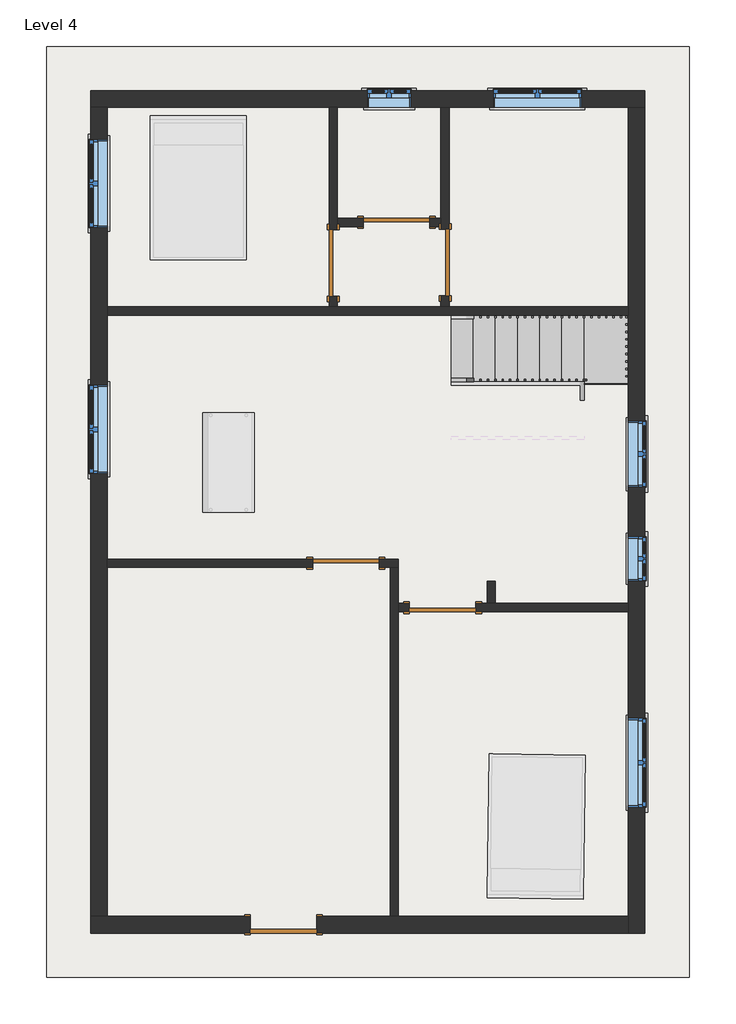
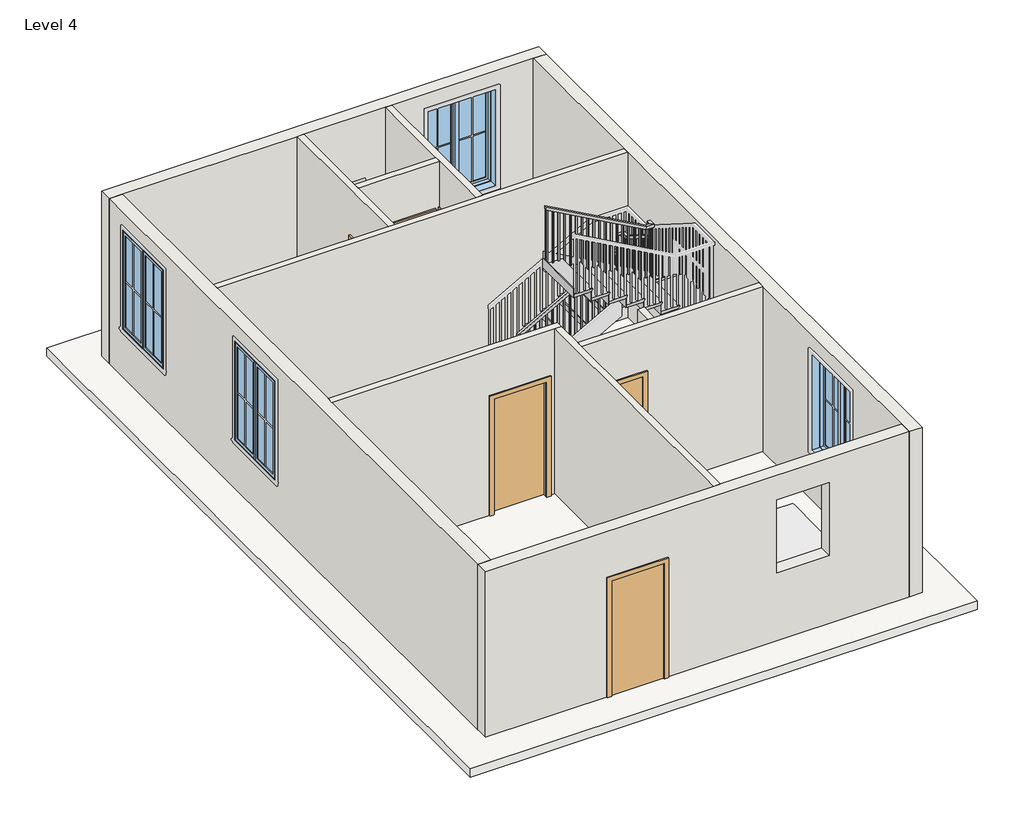
# One storey, part 1 of 2: 12 walls, 7 windows, 6 doors, 1 railing, 1 slab, 1 stair flight.
"""IFC4 building model written with IfcOpenShell, lengths in millimetres."""

from ifc_helpers import new_model, si_unit, frame, origin, place, context, project, spatial, polyline, outline, extrude, faceted_brep, transform, mapped, element, save
from components import door_e5f9f3c4, door_305aa2a5, door_0ca8825f, stair_flight_9a0573e1, window_c417fced, window_79f73a1a, window_6ca1769e

model = new_model("IFC4")

# Units and contexts
model_context = context("Model", 3, world=origin())
ifc_project = project(units=[si_unit("LENGTHUNIT", "METRE", prefix="MILLI")], contexts=[model_context])

# Site, building, storey
site = spatial("IfcSite", under=ifc_project)
building = spatial("IfcBuilding", under=site)
storey = spatial("IfcBuildingStorey", under=building, Name="Level 4", Elevation=9144.0)

# Doors
placement = place(None, origin())
door_shape = door_e5f9f3c4(model_context)
element("IfcDoor", 1, ObjectType="Single-Flush : 36\" x 84\"", at=placement, inside=storey, context=model_context, shape_type="MappedRepresentation", body=[
    mapped(door_shape, transform((5727.7, 12245.5823212, 9144.0), x_axis=(1.0, 0.0, 0.0), y_axis=(0.0, 1.0, 0.0), z_axis=(0.0, 0.0, 1.0))),
])
element("IfcDoor", 2, ObjectType="Single-Flush : 36\" x 84\"", at=placement, inside=storey, context=model_context, shape_type="MappedRepresentation", body=[
    mapped(door_shape, transform((6394.45, 11693.1323212, 9144.0), x_axis=(0.0, -1.0, 0.0), y_axis=(1.0, 0.0, 0.0), z_axis=(0.0, 0.0, 1.0))),
])
element("IfcDoor", 3, ObjectType="Single-Flush : 36\" x 84\"", at=placement, inside=storey, context=model_context, shape_type="MappedRepresentation", body=[
    mapped(door_shape, transform((6362.7, 6949.6823212, 9144.0), x_axis=(-1.0, 0.0, 0.0), y_axis=(0.0, -1.0, 0.0), z_axis=(0.0, 0.0, 1.0))),
])
element("IfcDoor", 4, ObjectType="Single-Flush : 36\" x 84\"", at=placement, inside=storey, context=model_context, shape_type="MappedRepresentation", body=[
    mapped(door_shape, transform((5029.2, 7559.2823212, 9144.0), x_axis=(1.0, 0.0, 0.0), y_axis=(0.0, 1.0, 0.0), z_axis=(0.0, 0.0, 1.0))),
])
door_2_shape = door_305aa2a5(model_context)
element("IfcDoor", 5, ObjectType="Single-Flush : 36\" x 84\"", at=placement, inside=storey, context=model_context, shape_type="MappedRepresentation", body=[
    mapped(door_2_shape, transform((4857.75, 11689.9573212, 9144.0), x_axis=(0.0, -1.0, 0.0), y_axis=(1.0, 0.0, 0.0), z_axis=(0.0, 0.0, 1.0))),
])
door_3_shape = door_0ca8825f(model_context)
element("IfcDoor", 6, ObjectType="Single-Flush : 36\" x 84\"", at=placement, inside=storey, context=model_context, shape_type="MappedRepresentation", body=[
    mapped(door_3_shape, transform((4171.95, 2587.2323212, 9144.0), x_axis=(-1.0, 0.0, 0.0), y_axis=(0.0, -1.0, 0.0), z_axis=(0.0, 0.0, 1.0))),
])

# Railing
element("IfcRailing", 7, ObjectType="Handrail - Rectangular", at=placement, inside=storey, context=model_context, shape_type="SolidModel", body=[
    faceted_brep([(6477.0, 10105.6323212, 10227.7333333), (6477.0, 10105.6323212, 10169.620221), (6477.0, 10054.8323212, 10169.620221), (6477.0, 10054.8323212, 10227.7333333), (8229.6, 10105.6323212, 11201.4), (8280.4, 10105.6323212, 11171.5091099), (8280.4, 10054.8323212, 11171.5091099), (8229.6, 10054.8323212, 11201.4), (8229.6, 10105.6323212, 11461.447619), (8280.4, 10105.6323212, 11410.647619), (8280.4, 10054.8323212, 11410.647619), (8229.6, 10054.8323212, 11461.447619), (8356.6, 10105.6323212, 11461.447619), (8356.6, 10105.6323212, 11410.647619), (8305.8, 10054.8323212, 11410.647619), (8305.8, 10054.8323212, 11461.447619), (8356.6, 9978.6323212, 11461.447619), (8356.6, 9963.8676405, 11410.647619), (8305.8, 9963.8676405, 11410.647619), (8305.8, 9978.6323212, 11461.447619), (8356.6, 9330.9323212, 11872.6857143), (8356.6, 9280.1323212, 11844.7652821), (8305.8, 9280.1323212, 11844.7652821), (8305.8, 9330.9323212, 11872.6857143), (8356.6, 9330.9323212, 12132.7333333), (8356.6, 9280.1323212, 12081.9333333), (8305.8, 9280.1323212, 12081.9333333), (8305.8, 9330.9323212, 12132.7333333), (8356.6, 9203.9323212, 12132.7333333), (8356.6, 9203.9323212, 12081.9333333), (8305.8, 9254.7323212, 12081.9333333), (8305.8, 9254.7323212, 12132.7333333), (8229.6, 9203.9323212, 12132.7333333), (8216.4363978, 9203.9323212, 12081.9333333), (8216.4363978, 9254.7323212, 12081.9333333), (8229.6, 9254.7323212, 12132.7333333), (6477.0, 9203.9323212, 13106.4), (6477.0, 9254.7323212, 13106.4), (6477.0, 9254.7323212, 13048.2868876), (6477.0, 9203.9323212, 13048.2868876)], [[[0, 1, 2, 3]], [[1, 0, 4, 5]], [[2, 1, 5, 6]], [[3, 2, 6, 7]], [[0, 3, 7, 4]], [[5, 4, 8, 9]], [[6, 5, 9, 10]], [[7, 6, 10, 11]], [[4, 7, 11, 8]], [[9, 8, 12, 13]], [[10, 9, 13, 14]], [[11, 10, 14, 15]], [[8, 11, 15, 12]], [[13, 12, 16, 17]], [[14, 13, 17, 18]], [[15, 14, 18, 19]], [[12, 15, 19, 16]], [[17, 16, 20, 21]], [[18, 17, 21, 22]], [[19, 18, 22, 23]], [[16, 19, 23, 20]], [[21, 20, 24, 25]], [[22, 21, 25, 26]], [[23, 22, 26, 27]], [[20, 23, 27, 24]], [[25, 24, 28, 29]], [[26, 25, 29, 30]], [[27, 26, 30, 31]], [[24, 27, 31, 28]], [[29, 28, 32, 33]], [[30, 29, 33, 34]], [[31, 30, 34, 35]], [[28, 31, 35, 32]], [[36, 37, 38, 39]], [[33, 32, 36, 39]], [[34, 33, 39, 38]], [[35, 34, 38, 37]], [[32, 35, 37, 36]]]),
    extrude(outline(polyline([(13028.8841099, 6511.925), (13039.4674432, 6492.875), (12022.6666667, 6492.875), (12022.6666667, 6511.925), (13028.8841099, 6511.925)])), frame((0.0, 9219.8073212, 0.0), z_axis=(0.0, 1.0, 0.0), x_axis=(0.0, 0.0, 1.0)), (0.0, 0.0, 1.0), 19.05),
    extrude(outline(polyline([(12972.4396654, 6613.525), (12983.0229988, 6594.475), (12022.6666667, 6594.475), (12022.6666667, 6613.525), (12972.4396654, 6613.525)])), frame((0.0, 9219.8073212, 0.0), z_axis=(0.0, 1.0, 0.0), x_axis=(0.0, 0.0, 1.0)), (0.0, 0.0, 1.0), 19.05),
    extrude(outline(polyline([(12915.995221, 6715.125), (12926.5785543, 6696.075), (12022.6666667, 6696.075), (12022.6666667, 6715.125), (12915.995221, 6715.125)])), frame((0.0, 9219.8073212, 0.0), z_axis=(0.0, 1.0, 0.0), x_axis=(0.0, 0.0, 1.0)), (0.0, 0.0, 1.0), 19.05),
    extrude(outline(polyline([(12859.5507765, 6816.725), (12870.1341099, 6797.675), (11853.3333333, 6797.675), (11853.3333333, 6816.725), (12859.5507765, 6816.725)])), frame((0.0, 9219.8073212, 0.0), z_axis=(0.0, 1.0, 0.0), x_axis=(0.0, 0.0, 1.0)), (0.0, 0.0, 1.0), 19.05),
    extrude(outline(polyline([(12803.1063321, 6918.325), (12813.6896654, 6899.275), (11853.3333333, 6899.275), (11853.3333333, 6918.325), (12803.1063321, 6918.325)])), frame((0.0, 9219.8073212, 0.0), z_axis=(0.0, 1.0, 0.0), x_axis=(0.0, 0.0, 1.0)), (0.0, 0.0, 1.0), 19.05),
    extrude(outline(polyline([(12746.6618876, 7019.925), (12757.245221, 7000.875), (11853.3333333, 7000.875), (11853.3333333, 7019.925), (12746.6618876, 7019.925)])), frame((0.0, 9219.8073212, 0.0), z_axis=(0.0, 1.0, 0.0), x_axis=(0.0, 0.0, 1.0)), (0.0, 0.0, 1.0), 19.05),
    extrude(outline(polyline([(12690.2174432, 7121.525), (12700.8007765, 7102.475), (11684.0, 7102.475), (11684.0, 7121.525), (12690.2174432, 7121.525)])), frame((0.0, 9219.8073212, 0.0), z_axis=(0.0, 1.0, 0.0), x_axis=(0.0, 0.0, 1.0)), (0.0, 0.0, 1.0), 19.05),
    extrude(outline(polyline([(12633.7729988, 7223.125), (12644.3563321, 7204.075), (11684.0, 7204.075), (11684.0, 7223.125), (12633.7729988, 7223.125)])), frame((0.0, 9219.8073212, 0.0), z_axis=(0.0, 1.0, 0.0), x_axis=(0.0, 0.0, 1.0)), (0.0, 0.0, 1.0), 19.05),
    extrude(outline(polyline([(12577.3285543, 7324.725), (12587.9118876, 7305.675), (11684.0, 7305.675), (11684.0, 7324.725), (12577.3285543, 7324.725)])), frame((0.0, 9219.8073212, 0.0), z_axis=(0.0, 1.0, 0.0), x_axis=(0.0, 0.0, 1.0)), (0.0, 0.0, 1.0), 19.05),
    extrude(outline(polyline([(12520.8841099, 7426.325), (12531.4674432, 7407.275), (11514.6666667, 7407.275), (11514.6666667, 7426.325), (12520.8841099, 7426.325)])), frame((0.0, 9219.8073212, 0.0), z_axis=(0.0, 1.0, 0.0), x_axis=(0.0, 0.0, 1.0)), (0.0, 0.0, 1.0), 19.05),
    extrude(outline(polyline([(12464.4396654, 7527.925), (12475.0229988, 7508.875), (11514.6666667, 7508.875), (11514.6666667, 7527.925), (12464.4396654, 7527.925)])), frame((0.0, 9219.8073212, 0.0), z_axis=(0.0, 1.0, 0.0), x_axis=(0.0, 0.0, 1.0)), (0.0, 0.0, 1.0), 19.05),
    extrude(outline(polyline([(12407.995221, 7629.525), (12418.5785543, 7610.475), (11514.6666667, 7610.475), (11514.6666667, 7629.525), (12407.995221, 7629.525)])), frame((0.0, 9219.8073212, 0.0), z_axis=(0.0, 1.0, 0.0), x_axis=(0.0, 0.0, 1.0)), (0.0, 0.0, 1.0), 19.05),
    extrude(outline(polyline([(12351.5507765, 7731.125), (12362.1341099, 7712.075), (11345.3333333, 7712.075), (11345.3333333, 7731.125), (12351.5507765, 7731.125)])), frame((0.0, 9219.8073212, 0.0), z_axis=(0.0, 1.0, 0.0), x_axis=(0.0, 0.0, 1.0)), (0.0, 0.0, 1.0), 19.05),
    extrude(outline(polyline([(12295.1063321, 7832.725), (12305.6896654, 7813.675), (11345.3333333, 7813.675), (11345.3333333, 7832.725), (12295.1063321, 7832.725)])), frame((0.0, 9219.8073212, 0.0), z_axis=(0.0, 1.0, 0.0), x_axis=(0.0, 0.0, 1.0)), (0.0, 0.0, 1.0), 19.05),
    extrude(outline(polyline([(12238.6618876, 7934.325), (12249.245221, 7915.275), (11345.3333333, 7915.275), (11345.3333333, 7934.325), (12238.6618876, 7934.325)])), frame((0.0, 9219.8073212, 0.0), z_axis=(0.0, 1.0, 0.0), x_axis=(0.0, 0.0, 1.0)), (0.0, 0.0, 1.0), 19.05),
    extrude(outline(polyline([(12182.2174432, 8035.925), (12192.8007765, 8016.875), (11176.0, 8016.875), (11176.0, 8035.925), (12182.2174432, 8035.925)])), frame((0.0, 9219.8073212, 0.0), z_axis=(0.0, 1.0, 0.0), x_axis=(0.0, 0.0, 1.0)), (0.0, 0.0, 1.0), 19.05),
    extrude(outline(polyline([(12125.7729988, 8137.525), (12136.3563321, 8118.475), (11176.0, 8118.475), (11176.0, 8137.525), (12125.7729988, 8137.525)])), frame((0.0, 9219.8073212, 0.0), z_axis=(0.0, 1.0, 0.0), x_axis=(0.0, 0.0, 1.0)), (0.0, 0.0, 1.0), 19.05),
    extrude(outline(polyline([(12069.3285543, 8239.125), (12079.9118876, 8220.075), (11176.0, 8220.075), (11176.0, 8239.125), (12069.3285543, 8239.125)])), frame((0.0, 9219.8073212, 0.0), z_axis=(0.0, 1.0, 0.0), x_axis=(0.0, 0.0, 1.0)), (0.0, 0.0, 1.0), 19.05),
    extrude(outline(polyline([(8321.675, 9276.9573212), (8340.725, 9276.9573212), (8340.725, 9257.9073212), (8321.675, 9257.9073212), (8321.675, 9276.9573212)])), frame((0.0, 0.0, 10837.3333333), z_axis=(0.0, 0.0, 1.0), x_axis=(1.0, 0.0, 0.0)), (0.0, 0.0, 1.0), 1244.6),
    extrude(outline(polyline([(9359.5073212, 11794.3684567), (9378.5573212, 11782.2732186), (9378.5573212, 10837.3333333), (9359.5073212, 10837.3333333), (9359.5073212, 11794.3684567)])), frame((8321.675, 0.0, 0.0), z_axis=(1.0, 0.0, 0.0), x_axis=(0.0, 1.0, 0.0)), (0.0, 0.0, 1.0), 19.05),
    extrude(outline(polyline([(9461.1073212, 11729.8605202), (9480.1573212, 11717.7652821), (9480.1573212, 10837.3333333), (9461.1073212, 10837.3333333), (9461.1073212, 11729.8605202)])), frame((8321.675, 0.0, 0.0), z_axis=(1.0, 0.0, 0.0), x_axis=(0.0, 1.0, 0.0)), (0.0, 0.0, 1.0), 19.05),
    extrude(outline(polyline([(9562.7073212, 11665.3525837), (9581.7573212, 11653.2573456), (9581.7573212, 10668.0), (9562.7073212, 10668.0), (9562.7073212, 11665.3525837)])), frame((8321.675, 0.0, 0.0), z_axis=(1.0, 0.0, 0.0), x_axis=(0.0, 1.0, 0.0)), (0.0, 0.0, 1.0), 19.05),
    extrude(outline(polyline([(9664.3073212, 11600.8446472), (9683.3573212, 11588.7494091), (9683.3573212, 10668.0), (9664.3073212, 10668.0), (9664.3073212, 11600.8446472)])), frame((8321.675, 0.0, 0.0), z_axis=(1.0, 0.0, 0.0), x_axis=(0.0, 1.0, 0.0)), (0.0, 0.0, 1.0), 19.05),
    extrude(outline(polyline([(9765.9073212, 11536.3367107), (9784.9573212, 11524.2414726), (9784.9573212, 10498.6666667), (9765.9073212, 10498.6666667), (9765.9073212, 11536.3367107)])), frame((8321.675, 0.0, 0.0), z_axis=(1.0, 0.0, 0.0), x_axis=(0.0, 1.0, 0.0)), (0.0, 0.0, 1.0), 19.05),
    extrude(outline(polyline([(9867.5073212, 11471.8287742), (9886.5573212, 11459.7335361), (9886.5573212, 10498.6666667), (9867.5073212, 10498.6666667), (9867.5073212, 11471.8287742)])), frame((8321.675, 0.0, 0.0), z_axis=(1.0, 0.0, 0.0), x_axis=(0.0, 1.0, 0.0)), (0.0, 0.0, 1.0), 19.05),
    extrude(outline(polyline([(9969.1073212, 11407.3208377), (9988.1573212, 11395.2255996), (9988.1573212, 10498.6666667), (9969.1073212, 10498.6666667), (9969.1073212, 11407.3208377)])), frame((8321.675, 0.0, 0.0), z_axis=(1.0, 0.0, 0.0), x_axis=(0.0, 1.0, 0.0)), (0.0, 0.0, 1.0), 19.05),
    extrude(outline(polyline([(8296.275, 10070.7073212), (8296.275, 10089.7573212), (8315.325, 10089.7573212), (8315.325, 10070.7073212), (8296.275, 10070.7073212)])), frame((0.0, 0.0, 10329.3333333), z_axis=(0.0, 0.0, 1.0), x_axis=(1.0, 0.0, 0.0)), (0.0, 0.0, 1.0), 1081.3142857),
    extrude(outline(polyline([(11134.4674432, 8213.725), (11123.8841099, 8194.675), (10160.0, 8194.675), (10160.0, 8213.725), (11134.4674432, 8213.725)])), frame((0.0, 10070.7073212, 0.0), z_axis=(0.0, 1.0, 0.0), x_axis=(0.0, 0.0, 1.0)), (0.0, 0.0, 1.0), 19.05),
    extrude(outline(polyline([(11078.0229988, 8112.125), (11067.4396654, 8093.075), (10160.0, 8093.075), (10160.0, 8112.125), (11078.0229988, 8112.125)])), frame((0.0, 10070.7073212, 0.0), z_axis=(0.0, 1.0, 0.0), x_axis=(0.0, 0.0, 1.0)), (0.0, 0.0, 1.0), 19.05),
    extrude(outline(polyline([(11021.5785543, 8010.525), (11010.995221, 7991.475), (10160.0, 7991.475), (10160.0, 8010.525), (11021.5785543, 8010.525)])), frame((0.0, 10070.7073212, 0.0), z_axis=(0.0, 1.0, 0.0), x_axis=(0.0, 0.0, 1.0)), (0.0, 0.0, 1.0), 19.05),
    extrude(outline(polyline([(10965.1341099, 7908.925), (10954.5507765, 7889.875), (9990.6666667, 7889.875), (9990.6666667, 7908.925), (10965.1341099, 7908.925)])), frame((0.0, 10070.7073212, 0.0), z_axis=(0.0, 1.0, 0.0), x_axis=(0.0, 0.0, 1.0)), (0.0, 0.0, 1.0), 19.05),
    extrude(outline(polyline([(10908.6896654, 7807.325), (10898.1063321, 7788.275), (9990.6666667, 7788.275), (9990.6666667, 7807.325), (10908.6896654, 7807.325)])), frame((0.0, 10070.7073212, 0.0), z_axis=(0.0, 1.0, 0.0), x_axis=(0.0, 0.0, 1.0)), (0.0, 0.0, 1.0), 19.05),
    extrude(outline(polyline([(10852.245221, 7705.725), (10841.6618876, 7686.675), (9990.6666667, 7686.675), (9990.6666667, 7705.725), (10852.245221, 7705.725)])), frame((0.0, 10070.7073212, 0.0), z_axis=(0.0, 1.0, 0.0), x_axis=(0.0, 0.0, 1.0)), (0.0, 0.0, 1.0), 19.05),
    extrude(outline(polyline([(10795.8007765, 7604.125), (10785.2174432, 7585.075), (9821.3333333, 7585.075), (9821.3333333, 7604.125), (10795.8007765, 7604.125)])), frame((0.0, 10070.7073212, 0.0), z_axis=(0.0, 1.0, 0.0), x_axis=(0.0, 0.0, 1.0)), (0.0, 0.0, 1.0), 19.05),
    extrude(outline(polyline([(10739.3563321, 7502.525), (10728.7729988, 7483.475), (9821.3333333, 7483.475), (9821.3333333, 7502.525), (10739.3563321, 7502.525)])), frame((0.0, 10070.7073212, 0.0), z_axis=(0.0, 1.0, 0.0), x_axis=(0.0, 0.0, 1.0)), (0.0, 0.0, 1.0), 19.05),
    extrude(outline(polyline([(10682.9118876, 7400.925), (10672.3285543, 7381.875), (9821.3333333, 7381.875), (9821.3333333, 7400.925), (10682.9118876, 7400.925)])), frame((0.0, 10070.7073212, 0.0), z_axis=(0.0, 1.0, 0.0), x_axis=(0.0, 0.0, 1.0)), (0.0, 0.0, 1.0), 19.05),
    extrude(outline(polyline([(10626.4674432, 7299.325), (10615.8841099, 7280.275), (9652.0, 7280.275), (9652.0, 7299.325), (10626.4674432, 7299.325)])), frame((0.0, 10070.7073212, 0.0), z_axis=(0.0, 1.0, 0.0), x_axis=(0.0, 0.0, 1.0)), (0.0, 0.0, 1.0), 19.05),
    extrude(outline(polyline([(10570.0229988, 7197.725), (10559.4396654, 7178.675), (9652.0, 7178.675), (9652.0, 7197.725), (10570.0229988, 7197.725)])), frame((0.0, 10070.7073212, 0.0), z_axis=(0.0, 1.0, 0.0), x_axis=(0.0, 0.0, 1.0)), (0.0, 0.0, 1.0), 19.05),
    extrude(outline(polyline([(10513.5785543, 7096.125), (10502.995221, 7077.075), (9652.0, 7077.075), (9652.0, 7096.125), (10513.5785543, 7096.125)])), frame((0.0, 10070.7073212, 0.0), z_axis=(0.0, 1.0, 0.0), x_axis=(0.0, 0.0, 1.0)), (0.0, 0.0, 1.0), 19.05),
    extrude(outline(polyline([(10457.1341099, 6994.525), (10446.5507765, 6975.475), (9482.6666667, 6975.475), (9482.6666667, 6994.525), (10457.1341099, 6994.525)])), frame((0.0, 10070.7073212, 0.0), z_axis=(0.0, 1.0, 0.0), x_axis=(0.0, 0.0, 1.0)), (0.0, 0.0, 1.0), 19.05),
    extrude(outline(polyline([(10400.6896654, 6892.925), (10390.1063321, 6873.875), (9482.6666667, 6873.875), (9482.6666667, 6892.925), (10400.6896654, 6892.925)])), frame((0.0, 10070.7073212, 0.0), z_axis=(0.0, 1.0, 0.0), x_axis=(0.0, 0.0, 1.0)), (0.0, 0.0, 1.0), 19.05),
    extrude(outline(polyline([(10344.245221, 6791.325), (10333.6618876, 6772.275), (9482.6666667, 6772.275), (9482.6666667, 6791.325), (10344.245221, 6791.325)])), frame((0.0, 10070.7073212, 0.0), z_axis=(0.0, 1.0, 0.0), x_axis=(0.0, 0.0, 1.0)), (0.0, 0.0, 1.0), 19.05),
    extrude(outline(polyline([(10287.8007765, 6689.725), (10277.2174432, 6670.675), (9313.3333333, 6670.675), (9313.3333333, 6689.725), (10287.8007765, 6689.725)])), frame((0.0, 10070.7073212, 0.0), z_axis=(0.0, 1.0, 0.0), x_axis=(0.0, 0.0, 1.0)), (0.0, 0.0, 1.0), 19.05),
    extrude(outline(polyline([(10231.3563321, 6588.125), (10220.7729988, 6569.075), (9313.3333333, 6569.075), (9313.3333333, 6588.125), (10231.3563321, 6588.125)])), frame((0.0, 10070.7073212, 0.0), z_axis=(0.0, 1.0, 0.0), x_axis=(0.0, 0.0, 1.0)), (0.0, 0.0, 1.0), 19.05),
    extrude(outline(polyline([(8321.675, 9238.8573212), (8340.725, 9238.8573212), (8340.725, 9219.8073212), (8321.675, 9219.8073212), (8321.675, 9238.8573212)])), frame((0.0, 0.0, 11006.6666667), z_axis=(0.0, 0.0, 1.0), x_axis=(1.0, 0.0, 0.0)), (0.0, 0.0, 1.0), 1075.2666667),
    extrude(outline(polyline([(8321.675, 10070.7073212), (8321.675, 10089.7573212), (8340.725, 10089.7573212), (8340.725, 10070.7073212), (8321.675, 10070.7073212)])), frame((0.0, 0.0, 10329.3333333), z_axis=(0.0, 0.0, 1.0), x_axis=(1.0, 0.0, 0.0)), (0.0, 0.0, 1.0), 1081.3142857),
    extrude(outline(polyline([(13037.7035543, 6496.05), (13048.2868876, 6477.0), (12022.6666667, 6477.0), (12022.6666667, 6496.05), (13037.7035543, 6496.05)])), frame((0.0, 9219.8073212, 0.0), z_axis=(0.0, 1.0, 0.0), x_axis=(0.0, 0.0, 1.0)), (0.0, 0.0, 1.0), 19.05),
    extrude(outline(polyline([(10180.2035543, 6496.05), (10169.620221, 6477.0), (9313.3333333, 6477.0), (9313.3333333, 6496.05), (10180.2035543, 6496.05)])), frame((0.0, 10070.7073212, 0.0), z_axis=(0.0, 1.0, 0.0), x_axis=(0.0, 0.0, 1.0)), (0.0, 0.0, 1.0), 19.05),
])

# Slab
element("IfcSlab", 8, ObjectType="Generic - 12\"", at=placement, inside=storey, context=model_context, shape_type="SweptSolid", body=[
    extrude(outline(polyline([(9753.6, 14664.9323212), (9753.6, 1863.3323212), (914.4, 1863.3323212), (914.4, 14664.9323212), (9753.6, 14664.9323212)])), frame((0.0, 0.0, 8991.6), z_axis=(0.0, 0.0, 1.0), x_axis=(1.0, 0.0, 0.0)), (0.0, 0.0, 1.0), 152.4),
])

# Stair flight
stair_flight_shape = stair_flight_9a0573e1(model_context)
element("IfcStairFlight", 9, ObjectType="2\" Tread 1\" Nosing 1/4\" Riser", at=placement, inside=storey, context=model_context, shape_type="MappedRepresentation", body=[
    mapped(stair_flight_shape, transform((0.0, 0.0, 0.0), x_axis=(1.0, 0.0, 0.0), y_axis=(0.0, 1.0, 0.0), z_axis=(0.0, 0.0, 1.0))),
])

# Walls
element("IfcWall", 10, ObjectType="Generic - 5\"", at=placement, inside=storey, context=model_context, shape_type="Brep", body=[
    faceted_brep([(4800.6, 11232.7573212, 11277.6), (4800.6, 11232.7573212, 9144.0), (4800.6, 11083.5323212, 9144.0), (4800.6, 11083.5323212, 12192.0), (4800.6, 13826.7323212, 12192.0), (4800.6, 13826.7323212, 9144.0), (4800.6, 12147.1573212, 9144.0), (4800.6, 12147.1573212, 11277.6), (4914.9, 11083.5323212, 9144.0), (4914.9, 11232.7573212, 9144.0), (4914.9, 11232.7573212, 11277.6), (4914.9, 12147.1573212, 11277.6), (4914.9, 12147.1573212, 9144.0), (4914.9, 12188.4323212, 9144.0), (4914.9, 12302.7323212, 9144.0), (4914.9, 13826.7323212, 9144.0), (4914.9, 13826.7323212, 12192.0), (4914.9, 12302.7323212, 12192.0), (4914.9, 12188.4323212, 12192.0), (4914.9, 11083.5323212, 12192.0)], [[[0, 1, 2, 3, 4, 5, 6, 7]], [[8, 9, 10, 11, 12, 13, 14, 15, 16, 17, 18, 19]], [[6, 5, 15, 14, 13, 12]], [[2, 1, 9, 8]], [[4, 3, 19, 18, 17, 16]], [[5, 4, 16, 15]], [[3, 2, 8, 19]], [[10, 9, 1, 0]], [[11, 10, 0, 7]], [[12, 11, 7, 6]]]),
])
element("IfcWall", 11, ObjectType="Generic - 5\"", at=placement, inside=storey, context=model_context, shape_type="Brep", body=[
    faceted_brep([(6337.3, 11235.9323212, 11277.6), (6337.3, 11235.9323212, 9144.0), (6337.3, 11083.5323212, 9144.0), (6337.3, 11083.5323212, 12192.0), (6337.3, 12188.4323212, 12192.0), (6337.3, 12302.7323212, 12192.0), (6337.3, 13826.7323212, 12192.0), (6337.3, 13826.7323212, 9144.0), (6337.3, 12302.7323212, 9144.0), (6337.3, 12188.4323212, 9144.0), (6337.3, 12150.3323212, 9144.0), (6337.3, 12150.3323212, 11277.6), (6451.6, 11083.5323212, 9144.0), (6451.6, 11235.9323212, 9144.0), (6451.6, 11235.9323212, 11277.6), (6451.6, 12150.3323212, 11277.6), (6451.6, 12150.3323212, 9144.0), (6451.6, 13826.7323212, 9144.0), (6451.6, 13826.7323212, 12192.0), (6451.6, 11083.5323212, 12192.0)], [[[0, 1, 2, 3, 4, 5, 6, 7, 8, 9, 10, 11]], [[12, 13, 14, 15, 16, 17, 18, 19]], [[2, 1, 13, 12]], [[10, 9, 8, 7, 17, 16]], [[6, 5, 4, 3, 19, 18]], [[7, 6, 18, 17]], [[3, 2, 12, 19]], [[14, 13, 1, 0]], [[15, 14, 0, 11]], [[16, 15, 11, 10]]]),
])
element("IfcWall", 12, ObjectType="Generic - 5\"", at=placement, inside=storey, context=model_context, shape_type="SweptSolid", body=[
    extrude(outline(polyline([(11277.6, 6184.9), (9144.0, 6184.9), (9144.0, 6337.3), (12192.0, 6337.3), (12192.0, 4914.9), (9144.0, 4914.9), (9144.0, 5270.5), (11277.6, 5270.5), (11277.6, 6184.9)])), frame((0.0, 12188.4323212, 0.0), z_axis=(0.0, 1.0, 0.0), x_axis=(0.0, 0.0, 1.0)), (0.0, 0.0, 1.0), 114.3),
])
element("IfcWall", 13, ObjectType="Generic - 5\"", at=placement, inside=storey, context=model_context, shape_type="Brep", body=[
    faceted_brep([(1752.6, 10969.2323212, 9144.0), (8915.4, 10969.2323212, 9144.0), (8915.4, 10969.2323212, 12192.0), (1752.6, 10969.2323212, 12192.0), (1752.6, 11083.5323212, 9144.0), (1752.6, 11083.5323212, 12192.0), (4800.6, 11083.5323212, 12192.0), (4914.9, 11083.5323212, 12192.0), (6337.3, 11083.5323212, 12192.0), (6451.6, 11083.5323212, 12192.0), (8915.4, 11083.5323212, 12192.0), (8915.4, 11083.5323212, 9144.0), (6451.6, 11083.5323212, 9144.0), (6337.3, 11083.5323212, 9144.0), (4914.9, 11083.5323212, 9144.0), (4800.6, 11083.5323212, 9144.0)], [[[0, 1, 2, 3]], [[4, 5, 6, 7, 8, 9, 10, 11, 12, 13, 14, 15]], [[1, 0, 4, 15, 14, 13, 12, 11]], [[3, 2, 10, 9, 8, 7, 6, 5]], [[2, 1, 11, 10]], [[0, 3, 5, 4]]]),
])
element("IfcWall", 14, ObjectType="Generic - 5\"", at=placement, inside=storey, context=model_context, shape_type="Brep", body=[
    faceted_brep([(5486.4, 7502.1323212, 11277.6), (5486.4, 7502.1323212, 9144.0), (5638.8, 7502.1323212, 9144.0), (5753.1, 7502.1323212, 9144.0), (5753.1, 7502.1323212, 12192.0), (5638.8, 7502.1323212, 12192.0), (1752.6, 7502.1323212, 12192.0), (1752.6, 7502.1323212, 9144.0), (4572.0, 7502.1323212, 9144.0), (4572.0, 7502.1323212, 11277.6), (5753.1, 7616.4323212, 9144.0), (5486.4, 7616.4323212, 9144.0), (5486.4, 7616.4323212, 11277.6), (4572.0, 7616.4323212, 11277.6), (4572.0, 7616.4323212, 9144.0), (1752.6, 7616.4323212, 9144.0), (1752.6, 7616.4323212, 12192.0), (5753.1, 7616.4323212, 12192.0)], [[[0, 1, 2, 3, 4, 5, 6, 7, 8, 9]], [[10, 11, 12, 13, 14, 15, 16, 17]], [[8, 7, 15, 14]], [[3, 2, 1, 11, 10]], [[6, 5, 4, 17, 16]], [[7, 6, 16, 15]], [[4, 3, 10, 17]], [[12, 11, 1, 0]], [[13, 12, 0, 9]], [[14, 13, 9, 8]]]),
])
element("IfcWall", 15, ObjectType="Generic - 5\"", at=placement, inside=storey, context=model_context, shape_type="Brep", body=[
    faceted_brep([(5638.8, 7502.1323212, 9144.0), (5638.8, 2701.5323212, 9144.0), (5638.8, 2701.5323212, 12192.0), (5638.8, 7502.1323212, 12192.0), (5753.1, 7502.1323212, 9144.0), (5753.1, 7502.1323212, 12192.0), (5753.1, 7006.8323212, 12192.0), (5753.1, 6892.5323212, 12192.0), (5753.1, 2701.5323212, 12192.0), (5753.1, 2701.5323212, 9144.0), (5753.1, 6892.5323212, 9144.0), (5753.1, 7006.8323212, 9144.0)], [[[0, 1, 2, 3]], [[4, 5, 6, 7, 8, 9, 10, 11]], [[1, 0, 4, 11, 10, 9]], [[3, 2, 8, 7, 6, 5]], [[0, 3, 5, 4]], [[2, 1, 9, 8]]]),
])
element("IfcWall", 16, ObjectType="Generic - 5\"", at=placement, inside=storey, context=model_context, shape_type="Brep", body=[
    faceted_brep([(5905.5, 7006.8323212, 11277.6), (5905.5, 7006.8323212, 9144.0), (5753.1, 7006.8323212, 9144.0), (5753.1, 7006.8323212, 12192.0), (6972.3, 7006.8323212, 12192.0), (7086.6, 7006.8323212, 12192.0), (8915.4, 7006.8323212, 12192.0), (8915.4, 7006.8323212, 9144.0), (7086.6, 7006.8323212, 9144.0), (6972.3, 7006.8323212, 9144.0), (6819.9, 7006.8323212, 9144.0), (6819.9, 7006.8323212, 11277.6), (5753.1, 6892.5323212, 9144.0), (5905.5, 6892.5323212, 9144.0), (5905.5, 6892.5323212, 11277.6), (6819.9, 6892.5323212, 11277.6), (6819.9, 6892.5323212, 9144.0), (8915.4, 6892.5323212, 9144.0), (8915.4, 6892.5323212, 12192.0), (5753.1, 6892.5323212, 12192.0)], [[[0, 1, 2, 3, 4, 5, 6, 7, 8, 9, 10, 11]], [[12, 13, 14, 15, 16, 17, 18, 19]], [[2, 1, 13, 12]], [[10, 9, 8, 7, 17, 16]], [[6, 5, 4, 3, 19, 18]], [[7, 6, 18, 17]], [[3, 2, 12, 19]], [[14, 13, 1, 0]], [[15, 14, 0, 11]], [[16, 15, 11, 10]]]),
])
element("IfcWall", 17, ObjectType="Generic - 5\"", at=placement, inside=storey, context=model_context, shape_type="SweptSolid", body=[
    extrude(outline(polyline([(7086.6, 7311.6323212), (7086.6, 7006.8323212), (6972.3, 7006.8323212), (6972.3, 7311.6323212), (7086.6, 7311.6323212)])), frame((0.0, 0.0, 9144.0), z_axis=(0.0, 0.0, 1.0), x_axis=(1.0, 0.0, 0.0)), (0.0, 0.0, 1.0), 3048.0),
])
element("IfcWall", 18, ObjectType="Generic - 8\"", at=placement, inside=storey, context=model_context, shape_type="Brep", body=[
    faceted_brep([(1524.0, 13826.7323212, 9144.0), (1752.6, 13826.7323212, 9144.0), (4800.6, 13826.7323212, 9144.0), (4914.9, 13826.7323212, 9144.0), (6337.3, 13826.7323212, 9144.0), (6451.6, 13826.7323212, 9144.0), (8915.4, 13826.7323212, 9144.0), (9144.0, 13826.7323212, 9144.0), (9144.0, 13826.7323212, 12192.0), (8915.4, 13826.7323212, 12192.0), (6451.6, 13826.7323212, 12192.0), (6337.3, 13826.7323212, 12192.0), (4914.9, 13826.7323212, 12192.0), (4800.6, 13826.7323212, 12192.0), (1752.6, 13826.7323212, 12192.0), (1524.0, 13826.7323212, 12192.0), (8274.05, 13826.7323212, 11887.2), (8274.05, 13826.7323212, 10058.4), (7054.85, 13826.7323212, 10058.4), (7054.85, 13826.7323212, 11887.2), (5930.9, 13826.7323212, 10972.8), (5930.9, 13826.7323212, 10058.4), (5321.3, 13826.7323212, 10058.4), (5321.3, 13826.7323212, 10972.8), (1524.0, 14055.3323212, 9144.0), (1524.0, 14055.3323212, 12192.0), (9144.0, 14055.3323212, 12192.0), (9144.0, 14055.3323212, 9144.0), (8274.05, 14055.3323212, 11887.2), (7054.85, 14055.3323212, 11887.2), (7054.85, 14055.3323212, 10058.4), (8274.05, 14055.3323212, 10058.4), (5930.9, 14055.3323212, 10972.8), (5321.3, 14055.3323212, 10972.8), (5321.3, 14055.3323212, 10058.4), (5930.9, 14055.3323212, 10058.4)], [[[0, 1, 2, 3, 4, 5, 6, 7, 8, 9, 10, 11, 12, 13, 14, 15], [16, 17, 18, 19], [20, 21, 22, 23]], [[24, 25, 26, 27], [28, 29, 30, 31], [32, 33, 34, 35]], [[7, 6, 5, 4, 3, 2, 1, 0, 24, 27]], [[8, 7, 27, 26]], [[0, 15, 25, 24]], [[17, 16, 28, 31]], [[18, 17, 31, 30]], [[19, 18, 30, 29]], [[16, 19, 29, 28]], [[21, 20, 32, 35]], [[22, 21, 35, 34]], [[23, 22, 34, 33]], [[20, 23, 33, 32]], [[15, 14, 13, 12, 11, 10, 9, 8, 26, 25]]]),
])
element("IfcWall", 19, ObjectType="Generic - 8\"", at=placement, inside=storey, context=model_context, shape_type="Brep", body=[
    faceted_brep([(8915.4, 13826.7323212, 9144.0), (8915.4, 11083.5323212, 9144.0), (8915.4, 10969.2323212, 9144.0), (8915.4, 7006.8323212, 9144.0), (8915.4, 6892.5323212, 9144.0), (8915.4, 2701.5323212, 9144.0), (8915.4, 2472.9323212, 9144.0), (8915.4, 2472.9323212, 12192.0), (8915.4, 2701.5323212, 12192.0), (8915.4, 6892.5323212, 12192.0), (8915.4, 7006.8323212, 12192.0), (8915.4, 10969.2323212, 12192.0), (8915.4, 11083.5323212, 12192.0), (8915.4, 13826.7323212, 12192.0), (8915.4, 4206.4823212, 11887.2), (8915.4, 4206.4823212, 10058.4), (8915.4, 5425.6823212, 10058.4), (8915.4, 5425.6823212, 11887.2), (8915.4, 7315.6010712, 10972.8), (8915.4, 7315.6010712, 10058.4), (8915.4, 7925.2010712, 10058.4), (8915.4, 7925.2010712, 10972.8), (8915.4, 8602.8899384, 11404.6), (8915.4, 8602.8899384, 10058.4), (8915.4, 9517.2899384, 10058.4), (8915.4, 9517.2899384, 11404.6), (9144.0, 13826.7323212, 9144.0), (9144.0, 13826.7323212, 12192.0), (9144.0, 2472.9323212, 12192.0), (9144.0, 2472.9323212, 9144.0), (9144.0, 4206.4823212, 11887.2), (9144.0, 5425.6823212, 11887.2), (9144.0, 5425.6823212, 10058.4), (9144.0, 4206.4823212, 10058.4), (9144.0, 7315.6010712, 10972.8), (9144.0, 7925.2010712, 10972.8), (9144.0, 7925.2010712, 10058.4), (9144.0, 7315.6010712, 10058.4), (9144.0, 8602.8899384, 11404.6), (9144.0, 9517.2899384, 11404.6), (9144.0, 9517.2899384, 10058.4), (9144.0, 8602.8899384, 10058.4)], [[[0, 1, 2, 3, 4, 5, 6, 7, 8, 9, 10, 11, 12, 13], [14, 15, 16, 17], [18, 19, 20, 21], [22, 23, 24, 25]], [[26, 27, 28, 29], [30, 31, 32, 33], [34, 35, 36, 37], [38, 39, 40, 41]], [[6, 5, 4, 3, 2, 1, 0, 26, 29]], [[0, 13, 27, 26]], [[7, 6, 29, 28]], [[15, 14, 30, 33]], [[16, 15, 33, 32]], [[17, 16, 32, 31]], [[14, 17, 31, 30]], [[19, 18, 34, 37]], [[20, 19, 37, 36]], [[21, 20, 36, 35]], [[18, 21, 35, 34]], [[23, 22, 38, 41]], [[24, 23, 41, 40]], [[25, 24, 40, 39]], [[22, 25, 39, 38]], [[13, 12, 11, 10, 9, 8, 7, 28, 27]]]),
])
element("IfcWall", 20, ObjectType="Generic - 8\"", at=placement, inside=storey, context=model_context, shape_type="Brep", body=[
    faceted_brep([(3714.75, 2701.5323212, 11277.6), (3714.75, 2701.5323212, 9144.0), (1752.6, 2701.5323212, 9144.0), (1524.0, 2701.5323212, 9144.0), (1524.0, 2701.5323212, 12192.0), (1752.6, 2701.5323212, 12192.0), (5638.8, 2701.5323212, 12192.0), (5753.1, 2701.5323212, 12192.0), (8915.4, 2701.5323212, 12192.0), (8915.4, 2701.5323212, 9144.0), (5753.1, 2701.5323212, 9144.0), (5638.8, 2701.5323212, 9144.0), (4629.15, 2701.5323212, 9144.0), (4629.15, 2701.5323212, 11277.6), (6610.35, 2701.5323212, 11738.3345423), (6610.35, 2701.5323212, 10392.1345423), (7524.75, 2701.5323212, 10392.1345423), (7524.75, 2701.5323212, 11738.3345423), (1524.0, 2472.9323212, 9144.0), (3714.75, 2472.9323212, 9144.0), (3714.75, 2472.9323212, 11277.6), (4629.15, 2472.9323212, 11277.6), (4629.15, 2472.9323212, 9144.0), (8915.4, 2472.9323212, 9144.0), (8915.4, 2472.9323212, 12192.0), (1524.0, 2472.9323212, 12192.0), (6610.35, 2472.9323212, 11738.3345423), (7524.75, 2472.9323212, 11738.3345423), (7524.75, 2472.9323212, 10392.1345423), (6610.35, 2472.9323212, 10392.1345423)], [[[0, 1, 2, 3, 4, 5, 6, 7, 8, 9, 10, 11, 12, 13], [14, 15, 16, 17]], [[18, 19, 20, 21, 22, 23, 24, 25], [26, 27, 28, 29]], [[3, 2, 1, 19, 18]], [[12, 11, 10, 9, 23, 22]], [[9, 8, 24, 23]], [[4, 3, 18, 25]], [[8, 7, 6, 5, 4, 25, 24]], [[20, 19, 1, 0]], [[21, 20, 0, 13]], [[22, 21, 13, 12]], [[15, 14, 26, 29]], [[16, 15, 29, 28]], [[17, 16, 28, 27]], [[14, 17, 27, 26]]]),
])
element("IfcWall", 21, ObjectType="Generic - 8\"", at=placement, inside=storey, context=model_context, shape_type="Brep", body=[
    faceted_brep([(1752.6, 2701.5323212, 9144.0), (1752.6, 7502.1323212, 9144.0), (1752.6, 7616.4323212, 9144.0), (1752.6, 10969.2323212, 9144.0), (1752.6, 11083.5323212, 9144.0), (1752.6, 13826.7323212, 9144.0), (1752.6, 13826.7323212, 12192.0), (1752.6, 11083.5323212, 12192.0), (1752.6, 10969.2323212, 12192.0), (1752.6, 7616.4323212, 12192.0), (1752.6, 7502.1323212, 12192.0), (1752.6, 2701.5323212, 12192.0), (1752.6, 13390.2194306, 11887.2), (1752.6, 13390.2194306, 10058.4), (1752.6, 12171.0194306, 10058.4), (1752.6, 12171.0194306, 11887.2), (1752.6, 10010.3823212, 11887.2), (1752.6, 10010.3823212, 10058.4), (1752.6, 8791.1823212, 10058.4), (1752.6, 8791.1823212, 11887.2), (1524.0, 2701.5323212, 9144.0), (1524.0, 2701.5323212, 12192.0), (1524.0, 13826.7323212, 12192.0), (1524.0, 13826.7323212, 9144.0), (1524.0, 13390.2194306, 11887.2), (1524.0, 12171.0194306, 11887.2), (1524.0, 12171.0194306, 10058.4), (1524.0, 13390.2194306, 10058.4), (1524.0, 10010.3823212, 11887.2), (1524.0, 8791.1823212, 11887.2), (1524.0, 8791.1823212, 10058.4), (1524.0, 10010.3823212, 10058.4)], [[[0, 1, 2, 3, 4, 5, 6, 7, 8, 9, 10, 11], [12, 13, 14, 15], [16, 17, 18, 19]], [[20, 21, 22, 23], [24, 25, 26, 27], [28, 29, 30, 31]], [[5, 4, 3, 2, 1, 0, 20, 23]], [[6, 5, 23, 22]], [[0, 11, 21, 20]], [[13, 12, 24, 27]], [[14, 13, 27, 26]], [[15, 14, 26, 25]], [[12, 15, 25, 24]], [[17, 16, 28, 31]], [[18, 17, 31, 30]], [[19, 18, 30, 29]], [[16, 19, 29, 28]], [[11, 10, 9, 8, 7, 6, 22, 21]]]),
])

# Windows
window_shape = window_c417fced(model_context)
element("IfcWindow", 22, ObjectType="Window-Casement-Double : 24\" x 36\"", at=placement, inside=storey, context=model_context, shape_type="MappedRepresentation", body=[
    mapped(window_shape, transform((9029.7, 7620.4010712, 9144.0), x_axis=(0.0, -1.0, 0.0), y_axis=(1.0, 0.0, 0.0), z_axis=(0.0, 0.0, 1.0))),
])
element("IfcWindow", 23, ObjectType="Window-Casement-Double : 24\" x 36\"", at=placement, inside=storey, context=model_context, shape_type="MappedRepresentation", body=[
    mapped(window_shape, transform((5626.1, 13941.0323212, 9144.0), x_axis=(1.0, 0.0, 0.0), y_axis=(0.0, 1.0, 0.0), z_axis=(0.0, 0.0, 1.0))),
])
window_2_shape = window_79f73a1a(model_context)
element("IfcWindow", 24, ObjectType="Window-Casement-Double : 36\" x 53\"", at=placement, inside=storey, context=model_context, shape_type="MappedRepresentation", body=[
    mapped(window_2_shape, transform((9029.7, 9060.0899384, 9144.0), x_axis=(0.0, -1.0, 0.0), y_axis=(1.0, 0.0, 0.0), z_axis=(0.0, 0.0, 1.0))),
])
window_3_shape = window_6ca1769e(model_context)
element("IfcWindow", 25, ObjectType="Window-Casement-Double : 48\" x 72\"", at=placement, inside=storey, context=model_context, shape_type="MappedRepresentation", body=[
    mapped(window_3_shape, transform((1638.3, 12780.6194306, 9144.0), x_axis=(0.0, 1.0, 0.0), y_axis=(-1.0, 0.0, 0.0), z_axis=(0.0, 0.0, 1.0))),
])
element("IfcWindow", 26, ObjectType="Window-Casement-Double : 48\" x 72\"", at=placement, inside=storey, context=model_context, shape_type="MappedRepresentation", body=[
    mapped(window_3_shape, transform((7664.45, 13941.0323212, 9144.0), x_axis=(1.0, 0.0, 0.0), y_axis=(0.0, 1.0, 0.0), z_axis=(0.0, 0.0, 1.0))),
])
element("IfcWindow", 27, ObjectType="Window-Casement-Double : 48\" x 72\"", at=placement, inside=storey, context=model_context, shape_type="MappedRepresentation", body=[
    mapped(window_3_shape, transform((9029.7, 4816.0823212, 9144.0), x_axis=(0.0, -1.0, 0.0), y_axis=(1.0, 0.0, 0.0), z_axis=(0.0, 0.0, 1.0))),
])
element("IfcWindow", 28, ObjectType="Window-Casement-Double : 48\" x 72\"", at=placement, inside=storey, context=model_context, shape_type="MappedRepresentation", body=[
    mapped(window_3_shape, transform((1638.3, 9400.7823212, 9144.0), x_axis=(0.0, 1.0, 0.0), y_axis=(-1.0, 0.0, 0.0), z_axis=(0.0, 0.0, 1.0))),
])

save(model, "model.ifc")

# Revit data of these elements
# Type "Single-Flush : 36\" x 84\""
#   Type Mark = "1"
#   Construction Type Id = "MDOOR"
#   Assembly Code = "C1020"
#   Analytic Construction = "Metal"
#   Thickness = 0' - 2"
#   Heat Transfer Coefficient (U) = 0.651978 BTU/(h·ft²·°F)
#   Height = 7' - 0"
#   Trim Projection Ext = 0' - 1"
#   Trim Projection Int = 0' - 1"
#   Trim Width = 0' - 3"
#   Width = 3' - 0"
#   Define Thermal Properties by = 1
#   Define Thermal Properties by = 1
#   Door Material = Door - Panel
#   Frame Material = Door - Frame
#   Visual Light Transmittance = 0
#   Solar Heat Gain Coefficient = 0
#   Function = (empty or 0)
#   Wall Closure = (empty or 0)
# Type "Handrail - Rectangular"
#   Assembly Code = "C2010400"
#   built-in parameter 1008612 = 0.0416667 (stored number, unit not read)
#   built-in parameter 1008611 = 0.0416667 (stored number, unit not read)
#   built-in parameter 1008609 = 0.333333 (stored number, unit not read)
#   built-in parameter 1008604 = 0.166667 (stored number, unit not read)
#   built-in parameter 1008603 = 0.166667 (stored number, unit not read)
#   Railing Height = 3' - 0"
#   built-in parameter 1008630 = 2
#   built-in parameter 1008610 = 2
#   built-in parameter 1008618 = Baluster - Square : 3/4"
# Type "Generic - 12\""
#   Assembly Code = "B1010"
#   Function = 0
#   Layers, outside or top first: 0' - 6" no material (function 1)
# Type "Generic - 5\""
#   Assembly Code = "B2010"
#   Layers, outside or top first: 0' - 4 1/2" no material (function 1)
# Type "Generic - 8\""
#   Assembly Code = "B2010"
#   Layers, outside or top first: 0' - 9" no material (function 1)
# Type "Window-Casement-Double : 24\" x 36\""
#   Type Mark = "14"
#   Fire Rating = "0.5h"
#   Assembly Code = "B2020100"
#   Analytic Construction = "Double glazing - domestic"
#   Frame Extension [instance default] = 0' - 0 1/4"
#   Window Inset [instance default] = 0' - 0"
#   Wall Thickness [instance default] = 0' - 6"
#   Interior Wall Closure [instance default] = 0' - 2 1/4"
#   Half Width = 1' - 0"
#   Visual Light Transmittance = 0.81
#   Thermal Resistance (R) = 1.8146 (h·ft²·°F)/BTU
#   Solar Heat Gain Coefficient = 0.76
#   Rough Width = 2' - 0 1/2"
#   Rough Height = 3' - 0 1/2"
#   Height = 3' - 0"
#   Heat Transfer Coefficient (U) = 0.5511 BTU/(h·ft²·°F)
#   Exterior Wall Closure [instance default] = 0' - 1 1/4"
#   Extension Jamb [instance default] = 0' - 2 1/4"
#   Default Sill Height = 3' - 0"
#   Width = 2' - 0"
#   Define Thermal Properties by = 0
#   Muntin Visibility = yes
#   Interior Trim Visibility [instance default] = yes
#   Exterior Trim Visibility [instance default] = yes
#   Extension Jamb Visibility [instance default] = yes
#   Interior Trim Material = Wood - Stained
#   Muntin Pattern = Muntin Pattern_2x2 : Muntin Pattern_2x2
#   Interior Trim = Trim-Window-Interior-Flat : Picture Frame
#   Interior Frame Material = Wood - Stained
#   Glass Panel Material = Glass
#   Exterior Trim Material = Clad - White
#   Exterior Trim = Trim-Window-Exterior-Flat : with Sill
#   Exterior Frame Material = Clad - White
#   Wall Closure = (empty or 0)
# Type "Window-Casement-Double : 36\" x 53\""
#   Type Mark = "15"
#   Fire Rating = "0.5h"
#   Assembly Code = "B2020100"
#   Analytic Construction = "Double glazing - domestic"
#   Frame Extension [instance default] = 0' - 0 1/4"
#   Window Inset [instance default] = 0' - 0"
#   Wall Thickness [instance default] = 0' - 6"
#   Interior Wall Closure [instance default] = 0' - 2 1/4"
#   Half Width = 1' - 6"
#   Visual Light Transmittance = 0.81
#   Thermal Resistance (R) = 1.8146 (h·ft²·°F)/BTU
#   Solar Heat Gain Coefficient = 0.76
#   Rough Width = 3' - 0 1/2"
#   Rough Height = 4' - 5 1/2"
#   Height = 4' - 5"
#   Heat Transfer Coefficient (U) = 0.5511 BTU/(h·ft²·°F)
#   Exterior Wall Closure [instance default] = 0' - 1 1/4"
#   Extension Jamb [instance default] = 0' - 2 1/4"
#   Default Sill Height = 3' - 0"
#   Width = 3' - 0"
#   Define Thermal Properties by = 0
#   Muntin Visibility = yes
#   Interior Trim Visibility [instance default] = yes
#   Exterior Trim Visibility [instance default] = yes
#   Extension Jamb Visibility [instance default] = yes
#   Interior Trim Material = Wood - Stained
#   Muntin Pattern = Muntin Pattern_2x2 : Muntin Pattern_2x2
#   Interior Trim = Trim-Window-Interior-Flat : Picture Frame
#   Interior Frame Material = Wood - Stained
#   Glass Panel Material = Glass
#   Exterior Trim Material = Clad - White
#   Exterior Trim = Trim-Window-Exterior-Flat : with Sill
#   Exterior Frame Material = Clad - White
#   Wall Closure = (empty or 0)
# Type "Window-Casement-Double : 48\" x 72\""
#   Type Mark = "17"
#   Fire Rating = "0.5h"
#   Assembly Code = "B2020100"
#   Analytic Construction = "Double glazing - domestic"
#   Frame Extension [instance default] = 0' - 0 1/4"
#   Window Inset [instance default] = 0' - 0"
#   Wall Thickness [instance default] = 0' - 6"
#   Interior Wall Closure [instance default] = 0' - 2 1/4"
#   Half Width = 2' - 0"
#   Visual Light Transmittance = 0.81
#   Thermal Resistance (R) = 1.8146 (h·ft²·°F)/BTU
#   Solar Heat Gain Coefficient = 0.76
#   Rough Width = 4' - 0 1/2"
#   Rough Height = 6' - 0 1/2"
#   Height = 6' - 0"
#   Heat Transfer Coefficient (U) = 0.5511 BTU/(h·ft²·°F)
#   Exterior Wall Closure [instance default] = 0' - 1 1/4"
#   Extension Jamb [instance default] = 0' - 2 1/4"
#   Default Sill Height = 3' - 0"
#   Width = 4' - 0"
#   Define Thermal Properties by = 0
#   Muntin Visibility = yes
#   Interior Trim Visibility [instance default] = yes
#   Exterior Trim Visibility [instance default] = yes
#   Extension Jamb Visibility [instance default] = yes
#   Interior Trim Material = Wood - Stained
#   Muntin Pattern = Muntin Pattern_2x2 : Muntin Pattern_2x2
#   Interior Trim = Trim-Window-Interior-Flat : Picture Frame
#   Interior Frame Material = Wood - Stained
#   Glass Panel Material = Glass
#   Exterior Trim Material = Clad - White
#   Exterior Trim = Trim-Window-Exterior-Flat : with Sill
#   Exterior Frame Material = Clad - White
#   Wall Closure = (empty or 0)
# Elements 1, 2, 3, 4, 5, 6 (IfcDoor, "Single-Flush : 36\" x 84\"")
#   Phase Created = New Construction
#   Materials on its faces: "Door - Frame", "Door - Panel"
# Element 7 (IfcRailing, "Handrail - Rectangular")
#   Phase Created = New Construction
# Element 8 (IfcSlab, "Generic - 12\"")
#   Height Offset From Level = 0' - 0"
#   Phase Created = New Construction
#   Materials on its faces: "Carpet (1)", "Clad - White"
# Element 9 (IfcStairFlight, "2\" Tread 1\" Nosing 1/4\" Riser")
#   Phase Created = New Construction
# Elements 10, 11, 12, 13, 14, 15, 16, 17 (IfcWall, "Generic - 5\"")
#   Top Offset = 0' - 0"
#   Base Offset = 0' - 0"
#   wall height = 10' - 0"
#   Phase Created = New Construction
#   Base Constraint = Level 4
#   Top Constraint = Level 5
#   Materials on its faces: "Default Wall"
# Elements 18, 19, 20, 21 (IfcWall, "Generic - 8\"")
#   Top Offset = 0' - 0"
#   Base Offset = 0' - 0"
#   Unconnected Height = 10' - 0"
#   wall height = 10' - 0"
#   Phase Created = New Construction
#   Base Constraint = Level 4
#   Materials on its faces: "Default Wall", "Wood - Stained"
# Element 22 (IfcWindow, "Window-Casement-Double : 24\" x 36\"")
#   Mark = "26"
#   Window Inset = 0' - 0"
#   Interior Wall Closure = 0' - 2 1/4"
#   Frame Extension = 0' - 0 1/4"
#   Exterior Wall Closure = 0' - 1 1/4"
#   Interior Trim Visibility = yes
#   Exterior Trim Visibility = yes
#   Phase Created = New Construction
#   Materials on its faces: "Wood - Stained", "Glass", "Clad - White"
# Element 23 (IfcWindow, "Window-Casement-Double : 24\" x 36\"")
#   Mark = "27"
#   Window Inset = 0' - 0"
#   Interior Wall Closure = 0' - 2 1/4"
#   Frame Extension = 0' - 0 1/4"
#   Exterior Wall Closure = 0' - 1 1/4"
#   Interior Trim Visibility = yes
#   Exterior Trim Visibility = yes
#   Phase Created = New Construction
#   Materials on its faces: "Wood - Stained", "Glass", "Clad - White"
# Element 24 (IfcWindow, "Window-Casement-Double : 36\" x 53\"")
#   Mark = "28"
#   Window Inset = 0' - 0"
#   Interior Wall Closure = 0' - 2 1/4"
#   Frame Extension = 0' - 0 1/4"
#   Exterior Wall Closure = 0' - 1 1/4"
#   Interior Trim Visibility = yes
#   Exterior Trim Visibility = yes
#   Phase Created = New Construction
#   Materials on its faces: "Wood - Stained", "Glass", "Clad - White"
# Element 25 (IfcWindow, "Window-Casement-Double : 48\" x 72\"")
#   Mark = "22"
#   Window Inset = 0' - 0"
#   Interior Wall Closure = 0' - 2 1/4"
#   Frame Extension = 0' - 0 1/4"
#   Exterior Wall Closure = 0' - 1 1/4"
#   Interior Trim Visibility = yes
#   Exterior Trim Visibility = yes
#   Phase Created = New Construction
#   Materials on its faces: "Wood - Stained", "Glass", "Clad - White"
# Element 26 (IfcWindow, "Window-Casement-Double : 48\" x 72\"")
#   Mark = "23"
#   Window Inset = 0' - 0"
#   Interior Wall Closure = 0' - 2 1/4"
#   Frame Extension = 0' - 0 1/4"
#   Exterior Wall Closure = 0' - 1 1/4"
#   Interior Trim Visibility = yes
#   Exterior Trim Visibility = yes
#   Phase Created = New Construction
#   Materials on its faces: "Wood - Stained", "Glass", "Clad - White"
# Element 27 (IfcWindow, "Window-Casement-Double : 48\" x 72\"")
#   Mark = "24"
#   Window Inset = 0' - 0"
#   Interior Wall Closure = 0' - 2 1/4"
#   Frame Extension = 0' - 0 1/4"
#   Exterior Wall Closure = 0' - 1 1/4"
#   Interior Trim Visibility = yes
#   Exterior Trim Visibility = yes
#   Phase Created = New Construction
#   Materials on its faces: "Wood - Stained", "Glass", "Clad - White"
# Element 28 (IfcWindow, "Window-Casement-Double : 48\" x 72\"")
#   Mark = "25"
#   Window Inset = 0' - 0"
#   Interior Wall Closure = 0' - 2 1/4"
#   Frame Extension = 0' - 0 1/4"
#   Exterior Wall Closure = 0' - 1 1/4"
#   Interior Trim Visibility = yes
#   Exterior Trim Visibility = yes
#   Phase Created = New Construction
#   Materials on its faces: "Wood - Stained", "Glass", "Clad - White"
# Materials
#   "Door - Panel": class "Wood", colour RGB 210 159 95, transparency 0, Cost = 0
#   "Door - Frame": colour RGB 118 70 51, transparency 0, Cost = 0
#   "Wood - Stained": class "Wood", colour RGB 224 178 126, transparency 0, Cost = 0
#   "Glass": class "Glass", colour RGB 0 128 192, transparency 0.75, Description = "Soda Lime Glass", Cost = 0
#   "Clad - White": class "Wood", colour RGB 242 242 238, transparency 0, Cost = 0
#   "Carpet (1)": class "Carpet", colour RGB 124 80 67, transparency 0, Description = "Interior finish", Cost = 0
#   "Default Wall": colour RGB 128 128 128, transparency 0, Cost = 0
